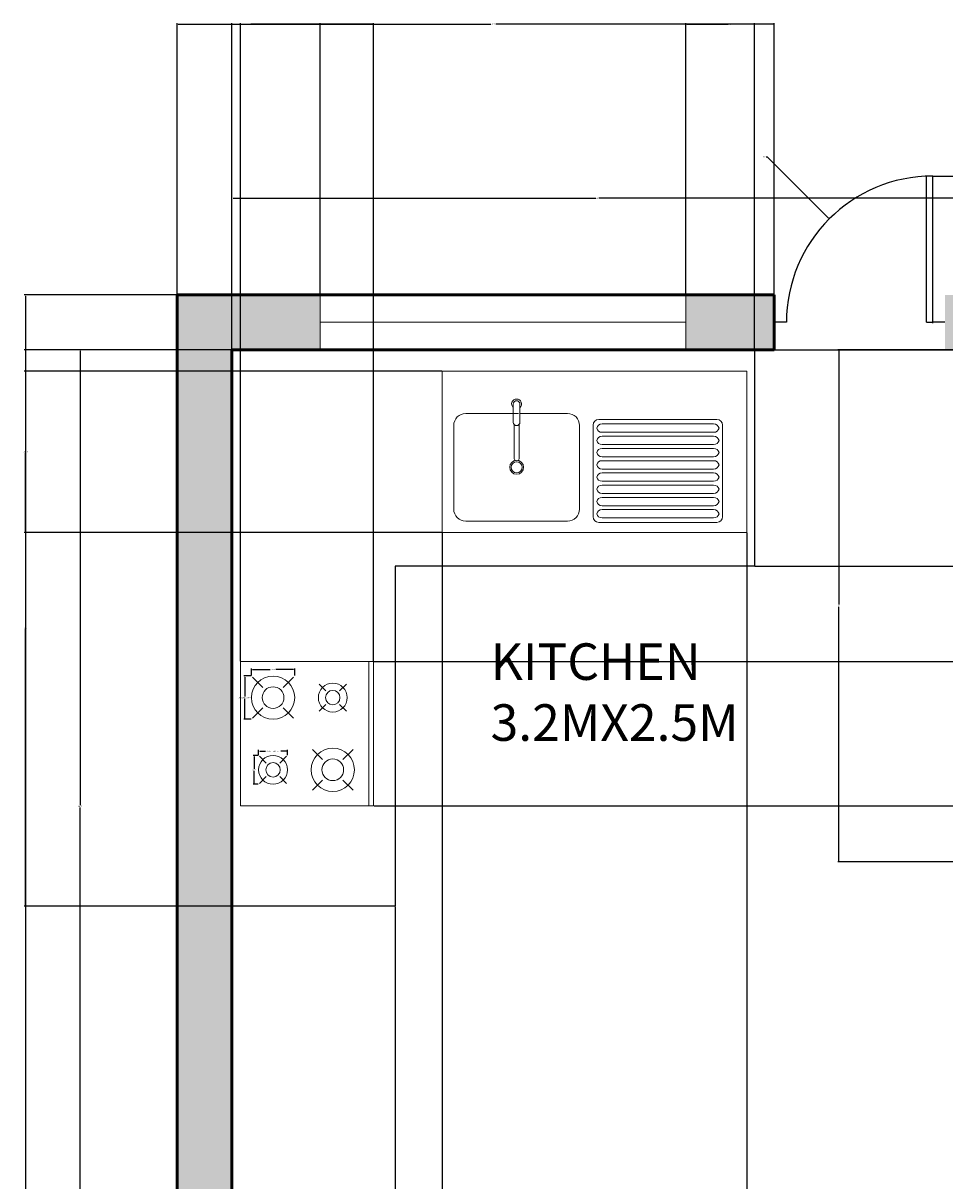
# Model space of a CAD drawing. Units: inches. Extents: x 3 to 380, y -485 to 60.
# Tile 7 of 8: x 3 to 154, y -130 to 60. Entities that reach past the tile are written whole.
import ezdxf

# ---------------------------------------------------------------- set-up
doc = ezdxf.new("R2010")
doc.units = ezdxf.units.IN
doc.header["$MEASUREMENT"] = 0
for name, color, linetype, lineweight in [('A-ANNO-DIMS', 2, 'Continuous', 18), ('A-AREA-IDEN', 7, 'Continuous', 25), ('A-DOOR', 3, 'Continuous', 25), ('A-EQPM', 9, 'Continuous', 18), ('A-FLOR-CASE', 8, 'Continuous', 25), ('A-FLOR-FIXT', 9, 'Continuous', 18), ('A-GLAZ', 4, 'Continuous', 18), ('A-WALL', 7, 'Continuous', 50), ('A-WALL-PATT', 252, 'Continuous', 13)]:
    doc.layers.add(name, color=color, linetype=linetype, lineweight=lineweight)
doc.styles.get("Standard").update_dxf_attribs({"font": 'arial.ttf'})
doc.dimstyles.get("Standard").update_dxf_attribs({"dimtxt": 0.18, "dimasz": 0.18, "dimexe": 0.18, "dimexo": 0.0625, "dimgap": 0.09, "dimtad": 0, "dimtih": 1, "dimtoh": 1, "dimdec": 0, "dimzin": 0, "dimdsep": 46, "dimlunit": 3, "dimtxsty": 'Standard', "dimcen": 0.09, "dimadec": 0, "dimazin": 0, "dimtfac": 1, "dimtdec": 0, "dimtofl": 0, "dimtmove": 0, "dimatfit": 3, "dimfxl": 1, "dimtolj": 1, "dimtzin": 0, "dimarcsym": 0})

# ---------------------------------------------------------------- blocks, each defined once
blk = doc.blocks.new('WIN-60X9')
for p, q in [((60, 9), (0, 9)), ((0, 9), (0, 0)), ((60, 0), (60, 9)), ((0, 4.5), (60, 4.5)), ((0, 0), (60, 0))]:
    blk.add_line(p, q)
blk = doc.blocks.new('DOOR-SWING-24')
for p, q in [((25, 0), (25, 24)), ((26, 0), (26, 24)), ((2, 0), (0, 0)), ((25, 0), (26, 0)), ((28, 0), (26, 0))]:
    blk.add_line(p, q)
blk.add_arc((26, 0), 24, 90, 180)
blk = doc.blocks.new('COOKTOP-BURNER-LARGE')
for p, q in [((1.88, 5.23), (0.2, 6.9)), ((5.23, 5.23), (6.9, 6.9)), ((1.88, 1.88), (0.2, 0.2)), ((5.23, 1.88), (6.9, 0.2))]:
    blk.add_line(p, q)
blk.add_circle((3.55, 3.55), 3.55)
for start, end in [(90, 270), (270, 90)]:
    blk.add_arc((3.55, 3.55), 1.78, start, end)
blk = doc.blocks.new('COOKTOP-BURNER-SMALL')
for p, q in [((1.25, 3.48), (0.14, 4.6)), ((3.48, 3.48), (4.6, 4.6)), ((1.25, 1.25), (0.14, 0.14)), ((3.48, 1.25), (4.6, 0.14))]:
    blk.add_line(p, q)
blk.add_circle((2.37, 2.37), 2.37)
for start, end in [(90, 270), (270, 90)]:
    blk.add_arc((2.37, 2.37), 1.18, start, end)
blk = doc.blocks.new('*D45')
at = {"layer": 'A-ANNO-DIMS', "color": 0, "lineweight": -2, "transparency": 16777216}
for p, q in [((39.97, -47.35), (38.78, -47.35)), ((38.96, -47.53), (38.96, -50.72)), ((38.96, -54.28), (38.96, -51.09)), ((39.97, -54.46), (38.78, -54.46))]:
    blk.add_line(p, q, dxfattribs=at)
at = {"layer": 'A-ANNO-DIMS', "color": 0, "transparency": 16777216}
for points in [[(38.93, -47.53), (38.99, -47.53), (38.96, -47.35)], [(38.93, -54.28), (38.99, -54.28), (38.96, -54.46)]]:
    blk.add_solid(points, dxfattribs=at)
at = {"layer": 'Defpoints', "color": 0, "transparency": 16777216}
for p in [(38.96, -47.35), (40.03, -47.35), (40.03, -54.46)]:
    blk.add_point(p, dxfattribs=at)
at = {"layer": 'A-ANNO-DIMS', "color": 0, "transparency": 16777216, "insert": (38.96, -50.91), "char_height": 0.18, "attachment_point": 5}
blk.add_mtext('\\A1;LARGE RING 7 TYP.', dxfattribs=at)
blk = doc.blocks.new('*D46')
at = {"layer": 'A-ANNO-DIMS', "color": 0, "lineweight": -2, "transparency": 16777216}
for p, q in [((40.03, -47.29), (40.03, -46.11)), ((40.21, -46.29), (43.12, -46.29)), ((46.95, -46.29), (44.04, -46.29)), ((47.13, -47.29), (47.13, -46.11))]:
    blk.add_line(p, q, dxfattribs=at)
at = {"layer": 'A-ANNO-DIMS', "color": 0, "transparency": 16777216}
for points in [[(40.21, -46.26), (40.21, -46.32), (40.03, -46.29)], [(46.95, -46.26), (46.95, -46.32), (47.13, -46.29)]]:
    blk.add_solid(points, dxfattribs=at)
at = {"layer": 'Defpoints', "color": 0, "transparency": 16777216}
for p in [(40.03, -47.35), (47.13, -46.29), (47.13, -47.35)]:
    blk.add_point(p, dxfattribs=at)
at = {"layer": 'A-ANNO-DIMS', "color": 0, "transparency": 16777216, "insert": (43.58, -46.29), "char_height": 0.18, "attachment_point": 5}
blk.add_mtext('\\A1;7 TYP.', dxfattribs=at)
blk = doc.blocks.new('*D47')
at = {"layer": 'A-ANNO-DIMS', "color": 0, "lineweight": -2, "transparency": 16777216}
for p, q in [((41.21, -60.32), (41.21, -59.49)), ((41.39, -59.67), (42.33, -59.67)), ((45.77, -59.67), (44.84, -59.67)), ((45.95, -60.32), (45.95, -59.49))]:
    blk.add_line(p, q, dxfattribs=at)
at = {"layer": 'A-ANNO-DIMS', "color": 0, "transparency": 16777216}
for points in [[(41.39, -59.64), (41.39, -59.7), (41.21, -59.67)], [(45.77, -59.64), (45.77, -59.7), (45.95, -59.67)]]:
    blk.add_solid(points, dxfattribs=at)
at = {"layer": 'Defpoints', "color": 0, "transparency": 16777216}
for p in [(41.21, -59.67), (41.21, -60.38), (45.95, -60.38)]:
    blk.add_point(p, dxfattribs=at)
at = {"layer": 'A-ANNO-DIMS', "color": 0, "transparency": 16777216, "insert": (43.58, -59.67), "char_height": 0.18, "attachment_point": 5}
blk.add_mtext('\\A1;SMALL RING 5 TYP.', dxfattribs=at)
blk = doc.blocks.new('*D48')
at = {"layer": 'A-ANNO-DIMS', "color": 0, "lineweight": -2, "transparency": 16777216}
for p, q in [((41.15, -60.38), (40.32, -60.38)), ((40.5, -60.56), (40.5, -62.57)), ((40.5, -64.94), (40.5, -62.93)), ((41.15, -65.12), (40.32, -65.12))]:
    blk.add_line(p, q, dxfattribs=at)
at = {"layer": 'A-ANNO-DIMS', "color": 0, "transparency": 16777216}
for points in [[(40.47, -60.56), (40.53, -60.56), (40.5, -60.38)], [(40.47, -64.94), (40.53, -64.94), (40.5, -65.12)]]:
    blk.add_solid(points, dxfattribs=at)
at = {"layer": 'Defpoints', "color": 0, "transparency": 16777216}
for p in [(41.21, -60.38), (40.5, -65.12), (41.21, -65.12)]:
    blk.add_point(p, dxfattribs=at)
at = {"layer": 'A-ANNO-DIMS', "color": 0, "transparency": 16777216, "insert": (40.5, -62.75), "char_height": 0.18, "attachment_point": 5}
blk.add_mtext('\\A1;5 TYP.', dxfattribs=at)
blk = doc.blocks.new('*D50')
at = {"layer": 'A-ANNO-DIMS', "color": 0, "lineweight": -2, "transparency": 16777216}
for p, q in [((27.78, 15.16), (2.76, 15.16)), ((2.94, 14.98), (2.94, -222.4)), ((2.94, -460.16), (2.94, -222.77)), ((27.78, -460.34), (2.76, -460.34))]:
    blk.add_line(p, q, dxfattribs=at)
at = {"layer": 'A-ANNO-DIMS', "color": 0, "transparency": 16777216}
for points in [[(2.91, 14.98), (2.97, 14.98), (2.94, 15.16)], [(2.91, -460.16), (2.97, -460.16), (2.94, -460.34)]]:
    blk.add_solid(points, dxfattribs=at)
at = {"layer": 'Defpoints', "color": 0, "transparency": 16777216}
for p in [(2.94, 15.16), (27.84, 15.16), (27.84, -460.34)]:
    blk.add_point(p, dxfattribs=at)
at = {"layer": 'A-ANNO-DIMS', "color": 0, "transparency": 16777216, "insert": (2.94, -222.59), "char_height": 0.18, "attachment_point": 5}
blk.add_mtext('\\A1;475.5', dxfattribs=at)
blk = doc.blocks.new('*D51')
at = {"layer": 'A-ANNO-DIMS', "color": 0, "lineweight": -2, "transparency": 16777216}
for p, q in [((151.9, 34.66), (379.92, 34.66)), ((379.74, 34.48), (379.74, -212.65)), ((379.74, -460.16), (379.74, -213.02)), ((354.9, -460.34), (379.92, -460.34))]:
    blk.add_line(p, q, dxfattribs=at)
at = {"layer": 'A-ANNO-DIMS', "color": 0, "transparency": 16777216}
for points in [[(379.71, 34.48), (379.77, 34.48), (379.74, 34.66)], [(379.71, -460.16), (379.77, -460.16), (379.74, -460.34)]]:
    blk.add_solid(points, dxfattribs=at)
at = {"layer": 'Defpoints', "color": 0, "transparency": 16777216}
for p in [(151.84, 34.66), (354.84, -460.34), (379.74, -460.34)]:
    blk.add_point(p, dxfattribs=at)
at = {"layer": 'A-ANNO-DIMS', "color": 0, "transparency": 16777216, "insert": (379.74, -212.84), "char_height": 0.18, "attachment_point": 5}
blk.add_mtext('\\A1;495', dxfattribs=at)
blk = doc.blocks.new('*D53')
at = {"layer": 'A-ANNO-DIMS', "color": 0, "lineweight": -2, "transparency": 16777216}
for p, q in [((36.78, 6.16), (11.76, 6.16)), ((11.94, 5.98), (11.94, -68.55)), ((11.94, -143.45), (11.94, -68.92)), ((36.78, -143.63), (11.76, -143.63))]:
    blk.add_line(p, q, dxfattribs=at)
at = {"layer": 'A-ANNO-DIMS', "color": 0, "transparency": 16777216}
for points in [[(11.91, 5.98), (11.97, 5.98), (11.94, 6.16)], [(11.91, -143.45), (11.97, -143.45), (11.94, -143.63)]]:
    blk.add_solid(points, dxfattribs=at)
at = {"layer": 'Defpoints', "color": 0, "transparency": 16777216}
for p in [(11.94, 6.16), (36.84, 6.16), (36.84, -143.63)]:
    blk.add_point(p, dxfattribs=at)
at = {"layer": 'A-ANNO-DIMS', "color": 0, "transparency": 16777216, "insert": (11.94, -68.73), "char_height": 0.18, "attachment_point": 5}
blk.add_mtext('\\A1;149.8', dxfattribs=at)
blk = doc.blocks.new('*D57')
at = {"layer": 'A-ANNO-DIMS', "color": 0, "lineweight": -2, "transparency": 16777216}
for p, q in [((27.84, 15.23), (27.84, 59.74)), ((28.02, 59.56), (39.26, 59.56)), ((51.16, 59.56), (39.92, 59.56)), ((51.34, 15.23), (51.34, 59.74))]:
    blk.add_line(p, q, dxfattribs=at)
at = {"layer": 'A-ANNO-DIMS', "color": 0, "transparency": 16777216}
for points in [[(28.02, 59.59), (28.02, 59.53), (27.84, 59.56)], [(51.16, 59.59), (51.16, 59.53), (51.34, 59.56)]]:
    blk.add_solid(points, dxfattribs=at)
at = {"layer": 'Defpoints', "color": 0, "transparency": 16777216}
for p in [(51.34, 59.56), (27.84, 15.16), (51.34, 15.16)]:
    blk.add_point(p, dxfattribs=at)
at = {"layer": 'A-ANNO-DIMS', "color": 0, "transparency": 16777216, "insert": (39.59, 59.56), "char_height": 0.18, "attachment_point": 5}
blk.add_mtext('\\A1;23.5', dxfattribs=at)
blk = doc.blocks.new('*D58')
at = {"layer": 'A-ANNO-DIMS', "color": 0, "lineweight": -2, "transparency": 16777216}
for p, q in [((111.34, 15.23), (111.34, 59.74)), ((111.52, 59.56), (118.27, 59.56)), ((125.66, 59.56), (118.91, 59.56)), ((125.84, 15.23), (125.84, 59.74))]:
    blk.add_line(p, q, dxfattribs=at)
at = {"layer": 'A-ANNO-DIMS', "color": 0, "transparency": 16777216}
for points in [[(111.52, 59.59), (111.52, 59.53), (111.34, 59.56)], [(125.66, 59.59), (125.66, 59.53), (125.84, 59.56)]]:
    blk.add_solid(points, dxfattribs=at)
at = {"layer": 'Defpoints', "color": 0, "transparency": 16777216}
for p in [(125.84, 59.56), (111.34, 15.16), (125.84, 15.16)]:
    blk.add_point(p, dxfattribs=at)
at = {"layer": 'A-ANNO-DIMS', "color": 0, "transparency": 16777216, "insert": (118.59, 59.56), "char_height": 0.18, "attachment_point": 5}
blk.add_mtext('\\A1;14.5', dxfattribs=at)
blk = doc.blocks.new('*D70')
at = {"layer": 'A-ANNO-DIMS', "color": 0, "lineweight": -2, "transparency": 16777216}
for p, q in [((36.84, 6.23), (36.84, 31.24)), ((37.02, 31.06), (96.56, 31.06)), ((156.66, 31.06), (97.12, 31.06)), ((156.84, 6.23), (156.84, 31.24))]:
    blk.add_line(p, q, dxfattribs=at)
at = {"layer": 'A-ANNO-DIMS', "color": 0, "transparency": 16777216}
for points in [[(37.02, 31.09), (37.02, 31.03), (36.84, 31.06)], [(156.66, 31.09), (156.66, 31.03), (156.84, 31.06)]]:
    blk.add_solid(points, dxfattribs=at)
at = {"layer": 'Defpoints', "color": 0, "transparency": 16777216}
for p in [(156.84, 31.06), (36.84, 6.16), (156.84, 6.16)]:
    blk.add_point(p, dxfattribs=at)
at = {"layer": 'A-ANNO-DIMS', "color": 0, "transparency": 16777216, "insert": (96.84, 31.06), "char_height": 0.18, "attachment_point": 5}
blk.add_mtext('\\A1;120', dxfattribs=at)
blk = doc.blocks.new('*D71')
at = {"layer": 'A-ANNO-DIMS', "color": 0, "lineweight": -2, "transparency": 16777216}
for p, q in [((161.28, 6.16), (136.26, 6.16)), ((136.44, 5.98), (136.44, -35.65)), ((136.44, -77.66), (136.44, -36.02)), ((161.28, -77.84), (136.26, -77.84))]:
    blk.add_line(p, q, dxfattribs=at)
at = {"layer": 'A-ANNO-DIMS', "color": 0, "transparency": 16777216}
for points in [[(136.41, 5.98), (136.47, 5.98), (136.44, 6.16)], [(136.41, -77.66), (136.47, -77.66), (136.44, -77.84)]]:
    blk.add_solid(points, dxfattribs=at)
at = {"layer": 'Defpoints', "color": 0, "transparency": 16777216}
for p in [(136.44, 6.16), (161.34, 6.16), (161.34, -77.84)]:
    blk.add_point(p, dxfattribs=at)
at = {"layer": 'A-ANNO-DIMS', "color": 0, "transparency": 16777216, "insert": (136.44, -35.84), "char_height": 0.18, "attachment_point": 5}
blk.add_mtext('\\A1;84', dxfattribs=at)
blk = doc.blocks.new('*D89')
at = {"layer": 'A-ANNO-DIMS', "color": 0, "lineweight": -2, "transparency": 16777216}
for p, q in [((36.84, 6.23), (36.84, 59.74)), ((37.02, 59.56), (79.34, 59.56)), ((122.44, 59.56), (80.13, 59.56)), ((122.62, 6.23), (122.62, 59.74))]:
    blk.add_line(p, q, dxfattribs=at)
at = {"layer": 'A-ANNO-DIMS', "color": 0, "transparency": 16777216}
for points in [[(37.02, 59.59), (37.02, 59.53), (36.84, 59.56)], [(122.44, 59.59), (122.44, 59.53), (122.62, 59.56)]]:
    blk.add_solid(points, dxfattribs=at)
at = {"layer": 'Defpoints', "color": 0, "transparency": 16777216}
for p in [(122.62, 59.56), (36.84, 6.16), (122.62, 6.16)]:
    blk.add_point(p, dxfattribs=at)
at = {"layer": 'A-ANNO-DIMS', "color": 0, "transparency": 16777216, "insert": (79.73, 59.56), "char_height": 0.18, "attachment_point": 5}
blk.add_mtext('\\A1;85.78', dxfattribs=at)
blk = doc.blocks.new('*D90')
at = {"layer": 'A-ANNO-DIMS', "color": 0, "lineweight": -2, "transparency": 16777216}
for p, q in [((36.78, 6.16), (2.76, 6.16)), ((2.94, 5.98), (2.94, -39.31)), ((2.94, -84.96), (2.94, -39.67)), ((36.78, -85.14), (2.76, -85.14))]:
    blk.add_line(p, q, dxfattribs=at)
at = {"layer": 'A-ANNO-DIMS', "color": 0, "transparency": 16777216}
for points in [[(2.91, 5.98), (2.97, 5.98), (2.94, 6.16)], [(2.91, -84.96), (2.97, -84.96), (2.94, -85.14)]]:
    blk.add_solid(points, dxfattribs=at)
at = {"layer": 'Defpoints', "color": 0, "transparency": 16777216}
for p in [(36.84, 6.16), (2.94, -85.14), (36.84, -85.14)]:
    blk.add_point(p, dxfattribs=at)
at = {"layer": 'A-ANNO-DIMS', "color": 0, "transparency": 16777216, "insert": (2.94, -39.49), "char_height": 0.18, "attachment_point": 5}
blk.add_mtext('\\A1;91.3', dxfattribs=at)
blk = doc.blocks.new('*D91')
at = {"layer": 'A-ANNO-DIMS', "color": 0, "lineweight": -2, "transparency": 16777216}
for p, q in [((122.68, 6.16), (379.92, 6.16)), ((379.74, 5.98), (379.74, -11.4)), ((379.74, -29.16), (379.74, -11.77)), ((122.68, -29.34), (379.92, -29.34))]:
    blk.add_line(p, q, dxfattribs=at)
at = {"layer": 'A-ANNO-DIMS', "color": 0, "transparency": 16777216}
for points in [[(379.71, 5.98), (379.77, 5.98), (379.74, 6.16)], [(379.71, -29.16), (379.77, -29.16), (379.74, -29.34)]]:
    blk.add_solid(points, dxfattribs=at)
at = {"layer": 'Defpoints', "color": 0, "transparency": 16777216}
for p in [(122.62, 6.16), (122.62, -29.34), (379.74, -29.34)]:
    blk.add_point(p, dxfattribs=at)
at = {"layer": 'A-ANNO-DIMS', "color": 0, "transparency": 16777216, "insert": (379.74, -11.59), "char_height": 0.18, "attachment_point": 5}
blk.add_mtext('\\A1;35.5', dxfattribs=at)
blk = doc.blocks.new('*D92')
at = {"layer": 'A-ANNO-DIMS', "color": 0, "lineweight": -2, "transparency": 16777216}
for p, q in [((36.84, -85.2), (36.84, -485.42)), ((63.65, -85.2), (63.65, -485.42)), ((37.02, -485.24), (49.87, -485.24)), ((63.47, -485.24), (50.62, -485.24))]:
    blk.add_line(p, q, dxfattribs=at)
at = {"layer": 'A-ANNO-DIMS', "color": 0, "transparency": 16777216}
for points in [[(37.02, -485.21), (37.02, -485.27), (36.84, -485.24)], [(63.47, -485.21), (63.47, -485.27), (63.65, -485.24)]]:
    blk.add_solid(points, dxfattribs=at)
at = {"layer": 'Defpoints', "color": 0, "transparency": 16777216}
for p in [(36.84, -85.14), (63.65, -85.14), (63.65, -485.24)]:
    blk.add_point(p, dxfattribs=at)
at = {"layer": 'A-ANNO-DIMS', "color": 0, "transparency": 16777216, "insert": (50.24, -485.24), "char_height": 0.18, "attachment_point": 5}
blk.add_mtext('\\A1;26.81', dxfattribs=at)
blk = doc.blocks.new('*D93')
at = {"layer": 'A-ANNO-DIMS', "color": 0, "lineweight": -2, "transparency": 16777216}
for p, q in [((71.32, -23.85), (71.32, -485.42)), ((121.32, -23.85), (121.32, -485.42)), ((71.5, -485.24), (95.92, -485.24)), ((121.14, -485.24), (96.72, -485.24))]:
    blk.add_line(p, q, dxfattribs=at)
at = {"layer": 'A-ANNO-DIMS', "color": 0, "transparency": 16777216}
for points in [[(71.5, -485.21), (71.5, -485.27), (71.32, -485.24)], [(121.14, -485.21), (121.14, -485.27), (121.32, -485.24)]]:
    blk.add_solid(points, dxfattribs=at)
at = {"layer": 'Defpoints', "color": 0, "transparency": 16777216}
for p in [(71.32, -23.79), (121.32, -23.79), (71.32, -485.24)]:
    blk.add_point(p, dxfattribs=at)
at = {"layer": 'A-ANNO-DIMS', "color": 0, "transparency": 16777216, "insert": (96.32, -485.24), "char_height": 0.18, "attachment_point": 5}
blk.add_mtext('\\A1;49.99', dxfattribs=at)
blk = doc.blocks.new('*D94')
at = {"layer": 'A-ANNO-DIMS', "color": 0, "lineweight": -2, "transparency": 16777216}
for p, q in [((71.26, 2.64), (2.76, 2.64)), ((2.94, 2.46), (2.94, -10.4)), ((2.94, -23.61), (2.94, -10.76)), ((71.26, -23.79), (2.76, -23.79))]:
    blk.add_line(p, q, dxfattribs=at)
at = {"layer": 'A-ANNO-DIMS', "color": 0, "transparency": 16777216}
for points in [[(2.91, 2.46), (2.97, 2.46), (2.94, 2.64)], [(2.91, -23.61), (2.97, -23.61), (2.94, -23.79)]]:
    blk.add_solid(points, dxfattribs=at)
at = {"layer": 'Defpoints', "color": 0, "transparency": 16777216}
for p in [(2.94, 2.64), (71.32, 2.64), (71.32, -23.79)]:
    blk.add_point(p, dxfattribs=at)
at = {"layer": 'A-ANNO-DIMS', "color": 0, "transparency": 16777216, "insert": (2.94, -10.58), "char_height": 0.18, "attachment_point": 5}
blk.add_mtext('\\A1;26.426', dxfattribs=at)
blk = doc.blocks.new('*D95')
at = {"layer": 'A-ANNO-DIMS', "color": 0, "lineweight": -2, "transparency": 16777216}
for p, q in [((38.23, -44.92), (38.23, 59.74)), ((38.41, 59.56), (48.69, 59.56)), ((59.91, 59.56), (49.62, 59.56)), ((60.09, -44.92), (60.09, 59.74))]:
    blk.add_line(p, q, dxfattribs=at)
at = {"layer": 'A-ANNO-DIMS', "color": 0, "transparency": 16777216}
for points in [[(38.41, 59.59), (38.41, 59.53), (38.23, 59.56)], [(59.91, 59.59), (59.91, 59.53), (60.09, 59.56)]]:
    blk.add_solid(points, dxfattribs=at)
at = {"layer": 'Defpoints', "color": 0, "transparency": 16777216}
for p in [(60.09, 59.56), (38.23, -44.99), (60.09, -44.99)]:
    blk.add_point(p, dxfattribs=at)
at = {"layer": 'A-ANNO-DIMS', "color": 0, "transparency": 16777216, "insert": (49.16, 59.56), "char_height": 0.18, "attachment_point": 5}
blk.add_mtext('\\A1;21.868', dxfattribs=at)
blk = doc.blocks.new('*D96')
at = {"layer": 'A-ANNO-DIMS', "color": 0, "lineweight": -2, "transparency": 16777216}
for p, q in [((60.16, -44.99), (379.92, -44.99)), ((379.74, -45.17), (379.74, -56.64)), ((379.74, -68.49), (379.74, -57.01)), ((60.16, -68.67), (379.92, -68.67))]:
    blk.add_line(p, q, dxfattribs=at)
at = {"layer": 'A-ANNO-DIMS', "color": 0, "transparency": 16777216}
for points in [[(379.71, -45.17), (379.77, -45.17), (379.74, -44.99)], [(379.71, -68.49), (379.77, -68.49), (379.74, -68.67)]]:
    blk.add_solid(points, dxfattribs=at)
at = {"layer": 'Defpoints', "color": 0, "transparency": 16777216}
for p in [(60.09, -44.99), (60.09, -68.67), (379.74, -68.67)]:
    blk.add_point(p, dxfattribs=at)
at = {"layer": 'A-ANNO-DIMS', "color": 0, "transparency": 16777216, "insert": (379.74, -56.83), "char_height": 0.18, "attachment_point": 5}
blk.add_mtext('\\A1;23.683', dxfattribs=at)
blk = doc.blocks.new('*D104')
at = {"layer": 'A-ANNO-DIMS', "color": 0, "lineweight": -2, "transparency": 16777216}
for p, q in [((124.51, 37.82), (124.69, 37.82)), ((124.69, 37.82), (134.74, 27.76)), ((151.75, 10.66), (151.93, 10.66)), ((151.84, 10.57), (151.84, 10.75))]:
    blk.add_line(p, q, dxfattribs=at)
at = {"layer": 'A-ANNO-DIMS', "color": 0, "transparency": 16777216}
blk.add_solid([(134.76, 27.78), (134.72, 27.74), (134.87, 27.64)], dxfattribs=at)
at = {"layer": 'Defpoints', "color": 0, "transparency": 16777216}
for p in [(134.87, 27.64), (151.84, 10.66)]:
    blk.add_point(p, dxfattribs=at)
at = {"layer": 'A-ANNO-DIMS', "color": 0, "transparency": 16777216, "insert": (124.2, 37.82), "char_height": 0.18, "attachment_point": 5}
blk.add_mtext('\\A1;R24', dxfattribs=at)

msp = doc.modelspace()

# ---------------------------------------------------------------- hatches: boundary and pattern name
at = {"layer": 'A-WALL-PATT'}
h = msp.add_hatch(color=256, dxfattribs=at)
h.dxf.hatch_style = 1
h.paths.add_polyline_path([(36.8404, 6.1643), (51.3404, 6.1643), (51.3404, 15.1643), (27.8404, 15.1643), (27.8404, -143.6318), (36.8404, -143.6318)])
h.paths.add_polyline_path([(125.8404, 10.6643), (125.8404, 15.1643), (111.3404, 15.1643), (111.3404, 6.1643), (125.8404, 6.1643)])
h.paths.add_polyline_path([(170.6358, 15.1643), (153.8404, 15.1643), (153.8404, 6.1643), (156.8404, 6.1643), (156.8404, -82.3357), (173.3404, -82.3357), (173.3404, -130.3357), (177.8404, -130.3357), (180.8404, -130.3357), (180.8404, -125.8357), (177.8404, -125.8357), (177.8404, -82.3357), (201.8404, -82.3357), (201.8404, -38.0857), (197.3404, -38.0857), (197.3404, -77.8357), (161.3404, -77.8357), (161.3404, 6.1643), (170.6358, 6.1643)])
h.paths.add_polyline_path([(241.3739, 15.1643), (194.6358, 15.1643), (194.6358, 6.1643), (241.3739, 6.1643)])
h.paths.add_polyline_path([(201.8404, 6.1643), (197.3404, 6.1643), (197.3404, -12.1977), (201.8404, -12.1977)], flags=17)
h.paths.add_polyline_path([(354.8404, 15.1643), (301.3739, 15.1643), (301.3739, 6.1643), (345.8404, 6.1643), (345.8404, -34.0336), (354.8404, -34.0336)])
h.paths.add_polyline_path([(354.8404, -94.0336), (345.8404, -94.0336), (345.8404, -159.3738), (354.8404, -159.3738)])
h.paths.add_polyline_path([(345.8404, -125.8357), (209.3404, -125.8357), (209.3404, -205.8357), (211.5904, -205.8357), (213.8404, -205.8357), (213.8404, -130.3357), (345.8404, -130.3357)])
h.paths.add_polyline_path([(36.8404, -203.6318), (27.8404, -203.6318), (27.8404, -270.1269), (36.8404, -270.1269)])
h.paths.add_polyline_path([(36.8404, -330.1269), (27.8404, -330.1269), (27.8404, -362.428), (57.3404, -362.428), (57.3404, -353.428), (36.8404, -353.428)])
h.paths.add_polyline_path([(177.8404, -331.3357), (180.8404, -331.3357), (180.8404, -326.8357), (173.3404, -326.8357), (173.3404, -353.428), (165.8404, -353.428), (165.8404, -362.428), (168.8404, -362.428), (168.8404, -451.3357), (168.8404, -460.3357), (231.8404, -460.3357), (231.8404, -451.3357), (177.8404, -451.3357)])
h.paths.add_polyline_path([(354.8404, -305.1003), (345.8404, -305.1003), (345.8404, -363.2829), (354.8404, -363.2829)])
h.paths.add_polyline_path([(345.8404, -326.8357), (213.8404, -326.8357), (213.8404, -312.8357), (211.5904, -312.8357), (209.3404, -312.8357), (209.3404, -331.3357), (345.8404, -331.3357)])
h.paths.add_polyline_path([(345.8404, -262.3357), (237.8404, -262.3357), (237.8404, -233.8357), (209.3404, -233.8357), (209.3404, -284.8357), (213.8404, -284.8357), (213.8404, -238.3357), (233.3404, -238.3357), (233.3404, -266.8357), (345.8404, -266.8357)])
h.paths.add_polyline_path([(354.8404, -219.3738), (345.8404, -219.3738), (345.8404, -281.1003), (354.8404, -281.1003)])

# ---------------------------------------------------------------- linework, layer by layer
at = {"layer": 'A-EQPM'}
for p, q in [((38.2256, -44.9851), (38.2256, -68.6686)), ((60.0933, -44.9851), (38.2256, -44.9851)), ((59.3038, -44.9851), (59.3038, -68.6686)), ((60.0933, -44.9851), (60.0933, -68.6686)), ((60.0933, -68.6686), (38.2256, -68.6686))]:
    msp.add_line(p, q, dxfattribs=at)
at = {"layer": 'A-FLOR-CASE'}
for p, q in [((122.6218, 6.1643), (122.6218, -29.3351)), ((122.6218, -29.3351), (63.6489, -29.3351)), ((63.6489, -29.3351), (63.6489, -62.1798)), ((63.6489, -62.1798), (63.6489, -85.1388)), ((63.6489, -85.1388), (36.8404, -85.1388))]:
    msp.add_line(p, q, dxfattribs=at)
at = {"layer": 'A-FLOR-FIXT'}
for p, q in [((71.3212, -23.7901), (71.3212, 2.636)), ((71.3212, 2.636), (121.3159, 2.636)), ((121.3159, 2.636), (121.3159, -23.7901)), ((83.8638, -4.2813), (75.2023, -4.2813)), ((91.917, -4.2813), (84.1064, -4.2813)), ((116.4387, -5.2846), (97.0314, -5.2846)), ((73.2341, -6.2496), (73.2341, -19.9832)), ((93.8853, -19.9832), (93.8853, -6.2496)), ((96.1202, -6.1958), (96.1202, -21.2393)), ((106.735, -6.0142), (97.579, -6.0142)), ((106.735, -7.3807), (97.579, -7.3807)), ((106.735, -6.0142), (115.8911, -6.0142)), ((106.735, -7.3807), (115.8911, -7.3807)), ((117.3499, -6.1958), (117.3499, -21.2393)), ((106.735, -8.0207), (97.579, -8.0207)), ((106.735, -9.3872), (97.579, -9.3872)), ((106.735, -8.0207), (115.8911, -8.0207)), ((106.735, -9.3872), (115.8911, -9.3872)), ((106.735, -10.0272), (97.579, -10.0272)), ((106.735, -11.3937), (97.579, -11.3937)), ((106.735, -10.0272), (115.8911, -10.0272)), ((106.735, -11.3937), (115.8911, -11.3937)), ((106.735, -12.0337), (97.579, -12.0337)), ((106.735, -12.0337), (115.8911, -12.0337)), ((106.735, -13.4001), (97.579, -13.4001)), ((106.735, -14.0402), (97.579, -14.0402)), ((106.735, -13.4001), (115.8911, -13.4001)), ((106.735, -14.0402), (115.8911, -14.0402)), ((106.735, -15.4066), (97.579, -15.4066)), ((106.735, -16.0466), (97.579, -16.0466)), ((106.735, -15.4066), (115.8911, -15.4066)), ((106.735, -16.0466), (115.8911, -16.0466)), ((106.735, -17.4131), (97.579, -17.4131)), ((106.735, -18.0531), (97.579, -18.0531)), ((106.735, -17.4131), (115.8911, -17.4131)), ((106.735, -18.0531), (115.8911, -18.0531)), ((106.735, -19.4196), (97.579, -19.4196)), ((106.735, -20.0596), (97.579, -20.0596)), ((106.735, -19.4196), (115.8911, -19.4196)), ((106.735, -20.0596), (115.8911, -20.0596)), ((75.2023, -21.9515), (91.917, -21.9515)), ((97.0314, -22.1506), (116.4387, -22.1506)), ((106.735, -21.4261), (97.579, -21.4261)), ((106.735, -21.4261), (115.8911, -21.4261)), ((71.3212, -23.7901), (121.3159, -23.7901))]:
    msp.add_line(p, q, dxfattribs=at)
for points in [[(83.0129, -2.7458), (83.0129, -5.749)], [(84.1064, -2.7458), (84.1064, -5.749)], [(83.1496, -6.0901), (83.1496, -11.6228)], [(83.9698, -6.0901), (83.9698, -11.6228)]]:
    msp.add_lwpolyline(points, dxfattribs=at)
for radius in [1.1391, 0.9112]:
    msp.add_circle((83.5597, -13.1164), radius, dxfattribs=at)
for centre, radius, start, end in [((83.5597, -2.7458), 0.8187, 311.901781, 228.098219), ((83.5597, -2.7458), 0.5467, 0, 180), ((75.2023, -6.2496), 1.9683, 90, 180), ((91.917, -6.2496), 1.9683, 0, 90), ((97.0314, -6.1958), 0.9112, 90, 180), ((116.4387, -6.1958), 0.9112, 0, 90), ((83.5597, -5.7278), 0.5472, 182.219765, 357.780235), ((97.579, -6.9255), 0.9112, 90, 165.509667), ((97.579, -6.4694), 0.9112, 194.490333, 270), ((115.8911, -6.9255), 0.9112, 14.490333, 90), ((115.8911, -6.4694), 0.9112, 270, 345.509667), ((97.579, -8.9319), 0.9112, 90, 165.509667), ((97.579, -8.4759), 0.9112, 194.490333, 270), ((115.8911, -8.9319), 0.9112, 14.490333, 90), ((115.8911, -8.4759), 0.9112, 270, 345.509667), ((97.579, -10.9384), 0.9112, 90, 165.509667), ((97.579, -10.4824), 0.9112, 194.490333, 270), ((115.8911, -10.9384), 0.9112, 14.490333, 90), ((115.8911, -10.4824), 0.9112, 270, 345.509667), ((83.5597, -11.6591), 0.4117, 174.94633, 5.05367), ((97.579, -12.9449), 0.9112, 90, 165.509667), ((97.579, -12.4889), 0.9112, 194.490333, 270), ((115.8911, -12.9449), 0.9112, 14.490333, 90), ((115.8911, -12.4889), 0.9112, 270, 345.509667), ((97.579, -14.9514), 0.9112, 90, 165.509667), ((97.579, -14.4954), 0.9112, 194.490333, 270), ((115.8911, -14.9514), 0.9112, 14.490333, 90), ((115.8911, -14.4954), 0.9112, 270, 345.509667), ((97.579, -16.9579), 0.9112, 90, 165.509667), ((97.579, -16.5019), 0.9112, 194.490333, 270), ((115.8911, -16.9579), 0.9112, 14.490333, 90), ((115.8911, -16.5019), 0.9112, 270, 345.509667), ((97.579, -18.9644), 0.9112, 90, 165.509667), ((97.579, -18.5084), 0.9112, 194.490333, 270), ((115.8911, -18.9644), 0.9112, 14.490333, 90), ((115.8911, -18.5084), 0.9112, 270, 345.509667), ((75.2023, -19.9832), 1.9683, 180, 270), ((91.917, -19.9832), 1.9683, 270, 0), ((97.579, -20.9709), 0.9112, 90, 165.509667), ((97.579, -20.5148), 0.9112, 194.490333, 270), ((115.8911, -20.9709), 0.9112, 14.490333, 90), ((115.8911, -20.5148), 0.9112, 270, 345.509667), ((97.0314, -21.2393), 0.9112, 180, 270), ((116.4387, -21.2393), 0.9112, 270, 0)]:
    msp.add_arc(centre, radius, start, end, dxfattribs=at)
at = {"layer": 'A-WALL'}
for p, q in [((27.8404, 15.1643), (27.8404, -460.3357)), ((27.8404, 15.1643), (125.8404, 15.1643)), ((125.8404, 10.6643), (125.8404, 15.1643)), ((125.8404, 10.6643), (125.8404, 6.1643)), ((36.8404, 6.1643), (125.8404, 6.1643)), ((36.8404, 6.1643), (36.8404, -353.428))]:
    msp.add_line(p, q, dxfattribs=at)

# ---------------------------------------------------------------- block references
at = {"layer": 'A-DOOR'}
msp.add_blockref('DOOR-SWING-24', (125.84, 10.664), dxfattribs=at)
at = {"layer": 'A-EQPM'}
for name, p in [('COOKTOP-BURNER-LARGE', (40.03, -54.458)), ('COOKTOP-BURNER-SMALL', (51.015, -53.274))]:
    msp.add_blockref(name, p, dxfattribs=at)
at = {"layer": 'A-EQPM', "rotation": 180}
for name, p in [('COOKTOP-BURNER-SMALL', (45.9501, -60.3797)), ('COOKTOP-BURNER-LARGE', (56.9351, -59.1957))]:
    msp.add_blockref(name, p, dxfattribs=at)
at = {"layer": 'A-GLAZ'}
msp.add_blockref('WIN-60X9', (51.3405, 6.164), dxfattribs=at)

# ---------------------------------------------------------------- texts
at = {"layer": 'A-AREA-IDEN', "insert": (79.2862, -41.9946), "char_height": 6, "attachment_point": 1}
msp.add_mtext('KITCHEN\\P3.2MX2.5M', dxfattribs=at)

# ---------------------------------------------------------------- dimensions: what is measured, and where the dimension line sits
at = {"layer": 'A-ANNO-DIMS'}
for base, p1, p2, override, picture, middle in [((51.3404, 59.5643), (27.8404, 15.1643), (51.3404, 15.1643), {"dimdec": 1, "dimlfac": 1, "dimrnd": 0, "dimzin": 0, "dimdsep": 46, "dimlunit": 2}, '*D57', (39.5904, 59.5643)), ((122.6218, 59.5643), (36.8404, 6.1643), (122.6218, 6.1643), {"dimdec": 2, "dimlfac": 1, "dimrnd": 0, "dimzin": 0, "dimdsep": 46, "dimlunit": 2}, '*D89', (79.7311, 59.5643)), ((60.0933, 59.5643), (38.2256, -44.9851), (60.0933, -44.9851), {"dimdec": 3, "dimlfac": 1, "dimrnd": 0, "dimzin": 0, "dimdsep": 46, "dimlunit": 2}, '*D95', (49.1594, 59.5643)), ((125.8404, 59.5643), (111.3404, 15.1643), (125.8404, 15.1643), {"dimdec": 1, "dimlfac": 1, "dimrnd": 0, "dimzin": 0, "dimdsep": 46, "dimlunit": 2}, '*D58', (118.5904, 59.5643)), ((156.8404, 31.0643), (36.8404, 6.1643), (156.8404, 6.1643), {"dimdec": 0, "dimlfac": 1, "dimrnd": 0, "dimzin": 0, "dimdsep": 46, "dimlunit": 2}, '*D70', (96.8404, 31.0643)), ((71.3212, -485.2357), (121.3159, -23.7901), (71.3212, -23.7901), {"dimdec": 2, "dimlfac": 1, "dimrnd": 0, "dimzin": 0, "dimdsep": 46, "dimlunit": 2}, '*D93', (96.3185, -485.2357)), ((63.6489, -485.2357), (36.8404, -85.1388), (63.6489, -85.1388), {"dimdec": 2, "dimlfac": 1, "dimrnd": 0, "dimzin": 0, "dimdsep": 46, "dimlunit": 2}, '*D92', (50.2446, -485.2357))]:
    dim = msp.add_linear_dim(base=base, p1=p1, p2=p2, dimstyle='Standard', override=override, dxfattribs=at)
    dim.commit()
    dim.dimension.update_dxf_attribs({"geometry": picture, "text_midpoint": middle})
dim = msp.add_radius_dim(center=(151.8404, 10.6643), mpoint=(134.87, 27.635), dimstyle='Standard', override={"dimdec": 0, "dimlfac": 1, "dimrnd": 0, "dimzin": 0, "dimdsep": 46, "dimlunit": 2}, dxfattribs=at)
dim.commit()
dim.dimension.update_dxf_attribs({"geometry": '*D104', "text_midpoint": (124.203, 37.8175), "dimtype": 164})
for base, p1, p2, override, picture, middle in [((379.7404, -460.3357), (151.8404, 34.6643), (354.8404, -460.3357), {"dimdec": 0, "dimlfac": 1, "dimrnd": 0, "dimzin": 0, "dimdsep": 46, "dimlunit": 2}, '*D51', (379.7404, -212.8357)), ((2.9404, 15.1643), (27.8404, -460.3357), (27.8404, 15.1643), {"dimdec": 1, "dimlfac": 1, "dimrnd": 0, "dimzin": 0, "dimdsep": 46, "dimlunit": 2}, '*D50', (2.9404, -222.5857)), ((2.9404, -85.1388), (36.8404, 6.1643), (36.8404, -85.1388), {"dimdec": 1, "dimlfac": 1, "dimrnd": 0, "dimzin": 0, "dimdsep": 46, "dimlunit": 2}, '*D90', (2.9404, -39.4872)), ((11.9404, 6.1643), (36.8404, -143.6318), (36.8404, 6.1643), {"dimdec": 1, "dimlfac": 1, "dimrnd": 0, "dimzin": 0, "dimdsep": 46, "dimlunit": 2}, '*D53', (11.9404, -68.7338)), ((379.7404, -29.3351), (122.6218, 6.1643), (122.6218, -29.3351), {"dimdec": 1, "dimlfac": 1, "dimrnd": 0, "dimzin": 0, "dimdsep": 46, "dimlunit": 2}, '*D91', (379.7404, -11.5854)), ((136.4404, 6.1643), (161.3404, -77.8357), (161.3404, 6.1643), {"dimdec": 0, "dimlfac": 1, "dimrnd": 0, "dimzin": 0, "dimdsep": 46, "dimlunit": 2}, '*D71', (136.4404, -35.8357)), ((2.9404, 2.636), (71.3212, -23.7901), (71.3212, 2.636), {"dimdec": 3, "dimlfac": 1, "dimrnd": 0, "dimzin": 0, "dimdsep": 46, "dimlunit": 2}, '*D94', (2.9404, -10.5771)), ((379.74035, -68.66856), (60.09329, -44.98511), (60.09329, -68.66856), {"dimdec": 3, "dimlfac": 1, "dimrnd": 0, "dimzin": 0, "dimdsep": 46, "dimlunit": 2}, '*D96', (379.74035, -56.82684))]:
    dim = msp.add_linear_dim(base=base, p1=p1, p2=p2, angle=90, dimstyle='Standard', override=override, dxfattribs=at)
    dim.commit()
    dim.dimension.update_dxf_attribs({"geometry": picture, "text_midpoint": middle})
for base, p1, p2, angle, text, picture, middle in [((38.9638, -47.3535), (40.0296, -54.4585), (40.0296, -47.3535), 90, 'LARGE RING <> TYP.', '*D45', (38.9638, -50.906)), ((40.5033, -65.116), (41.2138, -60.3794), (41.2138, -65.116), 270, '<> TYP.', '*D48', (40.5033, -62.7477)), ((41.2138, -59.6688), (45.9505, -60.3794), (41.2138, -60.3794), 180, 'SMALL RING <> TYP.', '*D47', (43.5821, -59.6688))]:
    dim = msp.add_linear_dim(base=base, p1=p1, p2=p2, angle=angle, text=text, dimstyle='Standard', override={"dimdec": 0, "dimlfac": 1, "dimrnd": 0, "dimzin": 0, "dimdsep": 46, "dimlunit": 2}, dxfattribs=at)
    dim.commit()
    dim.dimension.update_dxf_attribs({"geometry": picture, "text_midpoint": middle})
dim = msp.add_linear_dim(base=(47.1346, -46.2877), p1=(40.0296, -47.3535), p2=(47.1346, -47.3535), text='<> TYP.', dimstyle='Standard', override={"dimdec": 0, "dimlfac": 1, "dimrnd": 0, "dimzin": 0, "dimdsep": 46, "dimlunit": 2}, dxfattribs=at)
dim.commit()
dim.dimension.update_dxf_attribs({"geometry": '*D46', "text_midpoint": (43.5821, -46.2877)})

doc.saveas('drawing.dxf')
